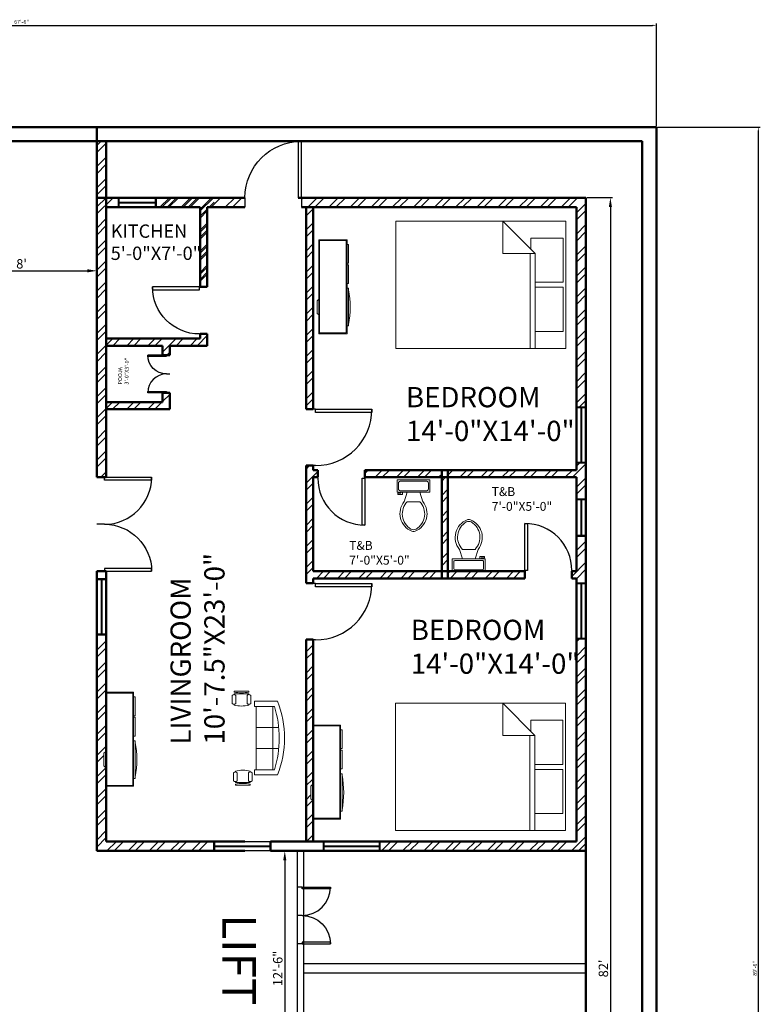
# Model space of a CAD drawing. Units: inches. Extents: x -12550 to 6516, y 1273 to 18700.
# Tile 11 of 19: x 3538 to 4010, y 1958 to 2587. Entities that reach past the tile are written whole.
import ezdxf

# ---------------------------------------------------------------- set-up
doc = ezdxf.new("R2010")
doc.units = ezdxf.units.IN
for name, color, linetype, lineweight in [('A-ANNO-DIMS', 2, 'Continuous', 18), ('A-AREA-IDEN', 1, 'Continuous', 18), ('A-DOOR', 5, 'Continuous', 25), ('A-EQPM', 4, 'Continuous', 25), ('A-FURN', 8, 'Continuous', 18), ('A-GLAZ', 3, 'Continuous', 25), ('A-WALL', 7, 'Continuous', 50), ('A-WALL-PATT', 8, 'Continuous', 13)]:
    doc.layers.add(name, color=color, linetype=linetype, lineweight=lineweight)
doc.styles.get("Standard").update_dxf_attribs({"font": 'arial.ttf'})
doc.dimstyles.new('ISO-25', dxfattribs={"dimtxt": 2.5, "dimasz": 2.5, "dimexe": 1.25, "dimexo": 0.625, "dimtad": 1, "dimlunit": 4, "dimtxsty": 'Standard', "dimcen": 2.5, "dimadec": 0, "dimazin": 0, "dimtfac": 1, "dimtmove": 0, "dimatfit": 3, "dimfxl": 1, "dimarcsym": 0})
pattern_1 = [(45, (1161.5385, 0), (-6.735192, 6.735192), []), (45, (1166.029, 0), (-6.735192, 6.735192), [])]
pattern_2 = [(45, (1161.5385, 567), (-6.735192, 6.735192), []), (45, (1166.029, 567), (-6.735192, 6.735192), [])]

# ---------------------------------------------------------------- blocks, each defined once
blk = doc.blocks.new('*U2')
for p, q in [((0, 0), (0, -5)), ((30, 0), (30, -5))]:
    blk.add_line(p, q)
blk.add_lwpolyline([(0, 0), (0, 30), (1.75, 30), (1.75, 0)], close=True)
blk.add_arc((0, 0), 30, 0, 90)
blk = doc.blocks.new('Bed - Queen')
for p, q in [((0, -80.00003), (0, 0)), ((0, 0), (59.99999, 0)), ((59.99999, 0), (59.99999, -80.00003)), ((7.99999, -1.2), (28.79998, -1.2)), ((7.99999, -14.4), (7.99999, -1.2)), ((28.79998, -1.2), (28.79998, -14.4)), ((31.19999, -1.2), (51.99999, -1.2)), ((31.19999, -14.4), (31.19999, -1.2)), ((51.99999, -1.2), (51.99999, -16.4)), ((0, -14.4), (44.8, -14.4)), ((44.8, -16.8), (0, -16.8)), ((59.99999, -29.6), (44.8, -14.4)), ((44.8, -14.4), (44.8, -29.6)), ((51.99999, -16.4), (46.79936, -16.4)), ((44.8, -29.6), (59.99999, -29.6)), ((59.99999, -80.00003), (0, -80.00003))]:
    blk.add_line(p, q)
blk = doc.blocks.new('Toilet - top')
for p, q in [((9.5, -6), (9.5, -2)), ((-10, -8.5), (-8, -8.5)), ((-10, -9.5), (-10, -8.5)), ((-7, -9.5), (-10, -9.5)), ((-8, -8.5), (-8, -8)), ((-7, -8), (-7, -9.5)), ((-4, -8), (-6, -14)), ((4, -8), (6, -14)), ((4, -14), (-4, -14))]:
    blk.add_line(p, q)
blk.add_lwpolyline([(10.5, -8), (10.5, 0), (-10.5, 0), (-10.5, -8)], close=True)
for points in [[(-9.5, -2), (-9.5, -6)], [(8.5, -1), (-8.5, -1)], [(-8.5, -7), (8.5, -7)]]:
    blk.add_lwpolyline(points)
for centre, radius, start, end in [((-8.62, -1.88), 0.884, 81.8699, 188.1301), ((-8.62, -6.12), 0.884, 171.8699, 278.1301), ((8.62, -1.88), 0.884, 351.8699, 98.1301), ((8.62, -6.12), 0.884, 261.8699, 8.1301), ((3.52, -21.58), 12.17, 141.46911, 247.97143), ((4.2, -21.82), 11.33, 136.36773, 238.94682), ((-3.52, -21.58), 12.17, 292.02843, 38.53071), ((-4.2, -21.82), 11.33, 301.05301, 43.63209), ((0, -27.88), 4, 245.73182, 294.26817), ((0, -29), 4, 254.86053, 285.13947)]:
    blk.add_arc(centre, radius, start, end)
blk = doc.blocks.new('Entertainment Center')
for p, q in [((-4, 0), (-5, -1)), ((4, 0), (-4, 0)), ((5, -1), (4, 0)), ((-17, -19), (-17, -1)), ((-17, -1), (43, -1)), ((-16.5, -18.5), (-16.5, -1.5)), ((-16.5, -1.5), (42.5, -1.5)), ((42.5, -1.5), (42.5, -18.5)), ((43, -1), (43, -19)), ((42.5, -18.5), (-16.5, -18.5)), ((43, -19), (-17, -19)), ((-12, -20), (-12, -19)), ((12, -20), (-12, -20)), ((12, -19), (12, -20)), ((15, -20), (15, -19)), ((27, -20), (15, -20)), ((27, -19), (27, -20)), ((28, -20), (28, -19)), ((40, -20), (28, -20)), ((40, -19), (40, -20))]:
    blk.add_line(p, q)
blk.add_arc((0, 40), 61, 259.6111, 280.3889)
blk = doc.blocks.new('Sofa - Roundback 7 ft.')
for p, q in [((-12.00002, -32.4421), (-12.00003, -6.5971)), ((11.99997, -32.4421), (11.99998, -6.5971)), ((-36.000027, -34), (-36.000027, -11.4696)), ((-35.999844, -13.3819), (35.9998, -13.3819)), ((35.99998, -34), (35.99998, -11.4696)), ((-36.000027, -32.4421), (35.99998, -32.4421))]:
    blk.add_line(p, q)
for points in [[(-36.000027, -34), (-42.000027, -34), (-42.000027, -8)], [(41.99998, -8), (41.99998, -34), (35.99998, -34)]]:
    blk.add_lwpolyline(points)
for centre, radius, start, end in [((0, -114.25), 114.25, 68.43141, 111.5686), ((-0.00001, -127.1968), 121.1968, 72.72033, 107.2797)]:
    blk.add_arc(centre, radius, start, end)
blk = doc.blocks.new('Chair - Desk')
for p, q in [((-8.5, 0), (-8.5, -1)), ((-8.5, 0), (8.5, 0)), ((8.5, 0), (8.5, -1)), ((-10.5, -5), (-10.5, -14)), ((-8.5, -3), (-8.5, -4)), ((-8.5, -3), (8.5, -3)), ((-6.5, -14), (-6.5, -5)), ((-2, -3), (-2, -1.9355)), ((2, -1.9576), (2, -3)), ((6.5, -5), (6.5, -14)), ((8.5, -3), (8.5, -4)), ((10.5, -14), (10.5, -5)), ((-8.5, -15), (-8.5, -16)), ((8.5, -15), (8.5, -16))]:
    blk.add_line(p, q)
for centre, radius, start, end in [((-8.5, -6.5), 2.5, 36.8699, 143.1301), ((0, 34.625), 36.625, 256.5803, 283.4197), ((8.5, -6.5), 2.5, 36.8699, 143.1301), ((-8.5, -12.5), 2.5, 216.8699, 323.1301), ((0, 19.625), 36.625, 256.5803, 283.4197), ((8.5, -12.5), 2.5, 216.8699, 323.1301)]:
    blk.add_arc(centre, radius, start, end)
blk = doc.blocks.new('*D28')
at = {"layer": 'A-ANNO-DIMS', "color": 0, "lineweight": -2, "transparency": 16777216}
for p, q in [((3714.6, 2056.25), (3705.89, 2056.25)), ((3707.14, 2050.25), (3707.14, 1912.25)), ((3714.6, 1906.25), (3705.89, 1906.25))]:
    blk.add_line(p, q, dxfattribs=at)
at = {"layer": 'A-ANNO-DIMS', "color": 0, "transparency": 16777216}
for points in [[(3706.14, 2050.25), (3708.14, 2050.25), (3707.14, 2056.25)], [(3706.14, 1912.25), (3708.14, 1912.25), (3707.14, 1906.25)]]:
    blk.add_solid(points, dxfattribs=at)
at = {"layer": 'Defpoints', "color": 0, "transparency": 16777216}
for p in [(3715.23, 2056.25), (3707.14, 1906.25), (3715.23, 1906.25)]:
    blk.add_point(p, dxfattribs=at)
at = {"layer": 'A-ANNO-DIMS', "color": 0, "transparency": 16777216, "insert": (3703.45, 1981.25), "char_height": 6, "attachment_point": 5, "rotation": 90}
blk.add_mtext('12\'-6"', dxfattribs=at)
blk = doc.blocks.new('*D30')
at = {"layer": 'A-ANNO-DIMS', "color": 0, "lineweight": -2, "transparency": 16777216}
for p, q in [((3899.85, 2473.25), (3916.1, 2473.25)), ((3914.85, 2467.25), (3914.85, 1495.25)), ((3899.85, 1489.25), (3916.1, 1489.25))]:
    blk.add_line(p, q, dxfattribs=at)
at = {"layer": 'A-ANNO-DIMS', "color": 0, "transparency": 16777216}
for points in [[(3913.85, 2467.25), (3915.85, 2467.25), (3914.85, 2473.25)], [(3913.85, 1495.25), (3915.85, 1495.25), (3914.85, 1489.25)]]:
    blk.add_solid(points, dxfattribs=at)
at = {"layer": 'Defpoints', "color": 0, "transparency": 16777216}
for p in [(3899.23, 2473.25), (3899.23, 1489.25), (3914.85, 1489.25)]:
    blk.add_point(p, dxfattribs=at)
at = {"layer": 'A-ANNO-DIMS', "color": 0, "transparency": 16777216, "insert": (3911.16, 1981.25), "char_height": 6, "attachment_point": 5, "rotation": 90}
blk.add_mtext("82'", dxfattribs=at)
blk = doc.blocks.new('*D27')
at = {"layer": 'A-ANNO-DIMS', "color": 0, "lineweight": -2, "transparency": 16777216}
for p, q in [((3491.23, 2407.12), (3491.23, 2427.81)), ((3497.23, 2426.56), (3581.23, 2426.56)), ((3587.23, 2407.12), (3587.23, 2427.81))]:
    blk.add_line(p, q, dxfattribs=at)
at = {"layer": 'A-ANNO-DIMS', "color": 0, "transparency": 16777216}
for points in [[(3497.23, 2427.56), (3497.23, 2425.56), (3491.23, 2426.56)], [(3581.23, 2427.56), (3581.23, 2425.56), (3587.23, 2426.56)]]:
    blk.add_solid(points, dxfattribs=at)
at = {"layer": 'Defpoints', "color": 0, "transparency": 16777216}
for p in [(3587.23, 2426.56), (3491.23, 2406.5), (3587.23, 2406.5)]:
    blk.add_point(p, dxfattribs=at)
at = {"layer": 'A-ANNO-DIMS', "color": 0, "transparency": 16777216, "insert": (3539.23, 2430.25), "char_height": 6, "attachment_point": 5}
blk.add_mtext("8'", dxfattribs=at)
blk = doc.blocks.new('WIN-3FT')
for p, q in [((0, 0), (0, 6)), ((0, 6), (36.02, 6)), ((36.02, 0), (0, 0)), ((0.5, 0), (0.5, 6)), ((35.52, 3.2), (0.5, 3.2)), ((35.52, 2.8), (0.5, 2.8)), ((35.52, 6), (35.52, 0)), ((36.02, 6), (36.02, 0))]:
    blk.add_line(p, q)
blk = doc.blocks.new('WIN-2FT')
for p, q in [((0, 0), (0, 24.02)), ((0, 24.02), (6, 24.02)), ((0, 23.52), (6, 23.52)), ((2.8, 0.5), (2.8, 23.52)), ((3.2, 0.5), (3.2, 23.52)), ((6, 24.02), (6, 0)), ((6, 0.5), (0, 0.5)), ((6, 0), (0, 0))]:
    blk.add_line(p, q)
blk = doc.blocks.new('*D103')
at = {"layer": 'A-ANNO-DIMS', "color": 0, "lineweight": -2, "transparency": 16777216}
for p, q in [((3134.23, 2518.87), (3134.23, 2584.5)), ((3136.73, 2583.25), (3941.73, 2583.25)), ((3944.23, 2518.87), (3944.23, 2584.5))]:
    blk.add_line(p, q, dxfattribs=at)
at = {"layer": 'A-ANNO-DIMS', "color": 0, "transparency": 16777216}
for points in [[(3136.73, 2583.66), (3136.73, 2582.83), (3134.23, 2583.25)], [(3941.73, 2583.66), (3941.73, 2582.83), (3944.23, 2583.25)]]:
    blk.add_solid(points, dxfattribs=at)
at = {"layer": 'Defpoints', "color": 0, "transparency": 16777216}
for p in [(3944.23, 2583.25), (3134.23, 2518.25), (3944.23, 2518.25)]:
    blk.add_point(p, dxfattribs=at)
at = {"layer": 'A-ANNO-DIMS', "color": 0, "transparency": 16777216, "insert": (3539.23, 2585.15), "char_height": 2.5, "attachment_point": 5}
blk.add_mtext('67\'-6"', dxfattribs=at)
blk = doc.blocks.new('*D104')
at = {"layer": 'A-ANNO-DIMS', "color": 0, "lineweight": -2, "transparency": 16777216}
for p, q in [((3944.85, 2518.25), (4010.48, 2518.25)), ((4009.23, 1446.75), (4009.23, 2515.75)), ((3944.85, 1444.25), (4010.48, 1444.25))]:
    blk.add_line(p, q, dxfattribs=at)
at = {"layer": 'A-ANNO-DIMS', "color": 0, "transparency": 16777216}
for points in [[(4008.81, 2515.75), (4009.64, 2515.75), (4009.23, 2518.25)], [(4008.81, 1446.75), (4009.64, 1446.75), (4009.23, 1444.25)]]:
    blk.add_solid(points, dxfattribs=at)
at = {"layer": 'Defpoints', "color": 0, "transparency": 16777216}
for p in [(3944.23, 2518.25), (4009.23, 2518.25), (3944.23, 1444.25)]:
    blk.add_point(p, dxfattribs=at)
at = {"layer": 'A-ANNO-DIMS', "color": 0, "transparency": 16777216, "insert": (4007.33, 1981.25), "char_height": 2.5, "attachment_point": 5, "rotation": 90}
blk.add_mtext('89\'-6"', dxfattribs=at)

msp = doc.modelspace()

# ---------------------------------------------------------------- hatches: boundary and pattern name
at = {"layer": 'A-WALL-PATT'}
h = msp.add_hatch(dxfattribs=at)
h.set_pattern_fill('ANSI32', color=256)
h.set_pattern_definition(pattern_1)
h.paths.add_polyline_path([(3593.227, 2509.247), (3587.227, 2509.247), (3587.227, 2473.247), (3593.227, 2473.247)])
h = msp.add_hatch(dxfattribs=at)
h.set_pattern_fill('ANSI32', color=256)
h.set_pattern_definition(pattern_2)
h.paths.add_polyline_path([(3600.985, 2473.247), (3587.227, 2473.247), (3587.227, 2294.747), (3592.227, 2294.747), (3593.227, 2294.747), (3593.227, 2467.247), (3600.985, 2467.247)])
h = msp.add_hatch(dxfattribs=at)
h.set_pattern_fill('ANSI32', color=256)
h.set_pattern_definition(pattern_1)
h.paths.add_polyline_path([(3625.002, 2473.247), (3625.002, 2467.247), (3653.227, 2467.247), (3653.227, 2416.247), (3657.727, 2416.247), (3657.727, 2467.247), (3681.727, 2467.247), (3681.727, 2473.247)])
h = msp.add_hatch(dxfattribs=at)
h.set_pattern_fill('ANSI32', color=256)
h.set_pattern_definition(pattern_2)
h.paths.add_polyline_path([(3662.066, 2473.247), (3625.002, 2473.247), (3625.002, 2467.247), (3653.227, 2467.247), (3653.227, 2416.247), (3657.727, 2416.247), (3657.727, 2467.247), (3662.066, 2467.247)])
h = msp.add_hatch(dxfattribs=at)
h.set_pattern_fill('ANSI32', color=256)
h.set_pattern_definition(pattern_2)
h.paths.add_polyline_path([(3717.727, 2473.247), (3717.727, 2467.247), (3893.227, 2467.247), (3893.227, 2339.747), (3899.227, 2339.747), (3899.227, 2473.247)])
h = msp.add_hatch(dxfattribs=at)
h.set_pattern_fill('ANSI32', color=256)
h.set_pattern_definition(pattern_2)
h.paths.add_polyline_path([(3725.227, 2467.247), (3720.727, 2467.247), (3720.727, 2338.247), (3725.227, 2338.247)])
h = msp.add_hatch(dxfattribs=at)
h.set_pattern_fill('ANSI32', color=256)
h.set_pattern_definition(pattern_2)
h.paths.add_polyline_path([(3657.727, 2386.247), (3653.227, 2386.247), (3653.227, 2383.247), (3593.227, 2383.247), (3593.227, 2378.747), (3629.227, 2378.747), (3629.227, 2372.747), (3631.727, 2372.747), (3633.727, 2372.747), (3633.727, 2378.747), (3657.727, 2378.747)])
h = msp.add_hatch(dxfattribs=at)
h.set_pattern_fill('ANSI32', color=256)
h.set_pattern_definition(pattern_2)
h.paths.add_polyline_path([(3633.727, 2348.747), (3631.727, 2348.747), (3629.227, 2348.747), (3629.227, 2342.747), (3593.227, 2342.747), (3593.227, 2338.247), (3633.727, 2338.247)])
h = msp.add_hatch(dxfattribs=at)
h.set_pattern_fill('ANSI32', color=256)
h.set_pattern_definition(pattern_2)
h.paths.add_polyline_path([(3725.227, 2294.747), (3728.227, 2294.747), (3728.227, 2299.247), (3725.227, 2299.247), (3725.227, 2302.247), (3720.727, 2302.247), (3720.727, 2227.247), (3725.227, 2227.247), (3725.227, 2230.247), (3728.18, 2230.247), (3807.227, 2230.247), (3807.227, 2234.747), (3728.18, 2234.747), (3725.227, 2234.747)])
h = msp.add_hatch(dxfattribs=at)
h.set_pattern_fill('ANSI32', color=256)
h.set_pattern_definition(pattern_2)
h.paths.add_polyline_path([(3899.227, 2303.73), (3893.227, 2303.73), (3893.227, 2299.247), (3890.227, 2299.247), (3811.227, 2299.247), (3811.227, 2294.747), (3890.227, 2294.747), (3893.227, 2294.747), (3893.227, 2281.042), (3899.227, 2281.042)])
h = msp.add_hatch(dxfattribs=at)
h.set_pattern_fill('ANSI32', color=256)
h.set_pattern_definition(pattern_2)
h.paths.add_polyline_path([(3807.227, 2299.247), (3758.227, 2299.247), (3758.227, 2294.747), (3807.227, 2294.747)], flags=17)
h = msp.add_hatch(dxfattribs=at)
h.set_pattern_fill('ANSI32', color=256)
h.set_pattern_definition(pattern_2)
h.paths.add_polyline_path([(3811.227, 2294.747), (3807.227, 2294.747), (3807.227, 2234.747), (3811.227, 2234.747)])
h = msp.add_hatch(dxfattribs=at)
h.set_pattern_fill('ANSI32', color=256)
h.set_pattern_definition(pattern_2)
h.paths.add_polyline_path([(3899.227, 2257.024), (3893.227, 2257.024), (3893.227, 2234.747), (3890.227, 2234.747), (3890.227, 2230.247), (3893.227, 2230.247), (3893.227, 2227.369), (3899.227, 2227.369)])
h = msp.add_hatch(dxfattribs=at)
h.set_pattern_fill('ANSI32', color=256)
h.set_pattern_definition(pattern_2)
h.paths.add_polyline_path([(3860.227, 2234.747), (3811.227, 2234.747), (3811.227, 2230.247), (3860.227, 2230.247)])
h = msp.add_hatch(dxfattribs=at)
h.set_pattern_fill('ANSI32', color=256)
h.set_pattern_definition(pattern_2)
h.paths.add_polyline_path([(3662.066, 2056.247), (3662.066, 2062.247), (3593.227, 2062.247), (3593.227, 2097.559), (3592.727, 2097.559), (3592.727, 2109.559), (3591.727, 2110.559), (3591.727, 2118.559), (3592.727, 2119.559), (3592.727, 2157.559), (3593.227, 2157.559), (3593.227, 2194.032), (3587.227, 2194.032), (3587.227, 2056.247)])
h = msp.add_hatch(dxfattribs=at)
h.set_pattern_fill('ANSI32', color=256)
h.set_pattern_definition(pattern_2)
h.paths.add_polyline_path([(3720.727, 2190.947), (3720.727, 2062.247), (3725.227, 2062.247), (3725.227, 2076.575), (3724.727, 2076.575), (3724.727, 2088.575), (3723.727, 2089.575), (3723.727, 2097.575), (3724.727, 2098.575), (3724.727, 2136.575), (3725.225, 2190.947)])
h = msp.add_hatch(dxfattribs=at)
h.set_pattern_fill('ANSI32', color=256)
h.set_pattern_definition(pattern_2)
h.paths.add_polyline_path([(3899.227, 2191.352), (3893.227, 2191.352), (3893.227, 2062.247), (3767.813, 2062.247), (3767.813, 2056.247), (3899.227, 2056.247)])

# ---------------------------------------------------------------- linework, layer by layer
at = {"layer": 'A-EQPM'}
for p, q in [((3715.227, 1906.247), (3715.227, 2056.247)), ((3899.227, 2056.247), (3715.227, 2056.247)), ((3719.227, 1906.247), (3719.227, 2056.247)), ((3899.227, 2056.247), (3899.227, 1906.247)), ((3899.227, 1984.247), (3719.227, 1984.247)), ((3899.227, 1978.247), (3719.227, 1978.247))]:
    msp.add_line(p, q, dxfattribs=at)
at = {"layer": 'A-WALL'}
for p, q in [((3134.227, 2518.247), (3944.227, 2518.247)), ((3587.227, 2294.747), (3587.227, 2518.247)), ((3944.227, 2518.247), (3944.227, 1444.247)), ((3143.227, 2509.247), (3935.227, 2509.247)), ((3715.627, 2509.247), (3415.627, 2509.247)), ((3593.227, 2294.747), (3593.227, 2509.247)), ((3935.227, 2509.247), (3935.227, 1453.247)), ((3681.727, 2473.247), (3587.227, 2473.247)), ((3720.727, 2473.247), (3715.627, 2473.247)), ((3899.227, 2473.247), (3720.727, 2473.247)), ((3899.227, 2060.923), (3899.227, 2473.247)), ((3653.227, 2467.247), (3593.227, 2467.247)), ((3653.227, 2416.247), (3653.227, 2467.247)), ((3681.727, 2467.247), (3657.727, 2467.247)), ((3657.727, 2416.247), (3657.727, 2467.247)), ((3720.727, 2467.247), (3717.727, 2467.247)), ((3893.227, 2467.247), (3720.727, 2467.247)), ((3720.727, 2338.247), (3720.727, 2467.247)), ((3725.227, 2338.247), (3725.227, 2467.247)), ((3893.227, 2299.247), (3893.227, 2467.247)), ((3653.227, 2416.247), (3657.727, 2416.247)), ((3653.227, 2383.247), (3593.227, 2383.247)), ((3653.227, 2383.247), (3653.227, 2386.247)), ((3657.727, 2386.247), (3653.227, 2386.247)), ((3657.727, 2378.747), (3657.727, 2386.247)), ((3657.727, 2383.247), (3657.727, 2386.247)), ((3629.227, 2378.747), (3593.227, 2378.747)), ((3629.227, 2372.747), (3629.227, 2378.747)), ((3657.727, 2378.747), (3633.727, 2378.747)), ((3633.727, 2372.747), (3633.727, 2378.747)), ((3629.227, 2372.747), (3633.727, 2372.747)), ((3629.227, 2342.747), (3629.227, 2348.747)), ((3633.727, 2348.747), (3629.227, 2348.747)), ((3633.727, 2338.247), (3633.727, 2348.747)), ((3633.727, 2342.747), (3633.727, 2348.747)), ((3629.227, 2342.747), (3593.227, 2342.747)), ((3633.727, 2338.247), (3593.227, 2338.247)), ((3720.727, 2338.247), (3725.227, 2338.247)), ((3720.727, 2227.247), (3720.727, 2302.247)), ((3725.227, 2302.247), (3720.727, 2302.247)), ((3725.227, 2299.247), (3725.227, 2302.247)), ((3725.227, 2299.247), (3725.227, 2302.247)), ((3725.227, 2299.247), (3725.227, 2302.247)), ((3725.227, 2299.247), (3725.227, 2302.247)), ((3593.227, 2294.747), (3587.227, 2294.747)), ((3728.227, 2299.247), (3725.227, 2299.247)), ((3728.227, 2294.747), (3725.227, 2294.747)), ((3725.227, 2234.747), (3725.227, 2294.747)), ((3725.227, 2234.747), (3725.227, 2294.747)), ((3725.227, 2234.747), (3725.227, 2294.747)), ((3725.227, 2294.747), (3728.227, 2294.747)), ((3728.227, 2294.747), (3728.227, 2299.247)), ((3890.227, 2299.247), (3758.227, 2299.247)), ((3758.227, 2299.247), (3758.227, 2294.747)), ((3890.227, 2294.747), (3758.227, 2294.747)), ((3807.227, 2230.247), (3807.227, 2299.247)), ((3811.227, 2230.247), (3811.227, 2299.247)), ((3893.227, 2299.247), (3890.227, 2299.247)), ((3893.227, 2299.247), (3890.227, 2299.247)), ((3893.227, 2294.747), (3890.227, 2294.747)), ((3893.227, 2234.747), (3893.227, 2294.747)), ((3593.227, 2234.747), (3587.227, 2234.747)), ((3587.227, 2056.247), (3587.227, 2234.747)), ((3593.227, 2062.247), (3593.227, 2234.747)), ((3728.18, 2234.747), (3725.227, 2234.747)), ((3860.227, 2234.747), (3728.18, 2234.747)), ((3860.227, 2234.747), (3860.227, 2230.247)), ((3893.227, 2234.747), (3890.227, 2234.747)), ((3890.227, 2230.247), (3890.227, 2234.747)), ((3720.727, 2230.247), (3720.727, 2227.247)), ((3720.727, 2227.247), (3725.227, 2227.247)), ((3728.18, 2230.247), (3725.227, 2230.247)), ((3725.227, 2227.247), (3725.227, 2230.247)), ((3725.227, 2227.247), (3725.227, 2230.247)), ((3725.227, 2227.247), (3725.227, 2230.247)), ((3860.227, 2230.247), (3728.18, 2230.247)), ((3893.227, 2230.247), (3890.227, 2230.247)), ((3893.227, 2230.247), (3890.227, 2230.247)), ((3893.227, 2062.247), (3893.227, 2230.247)), ((3720.727, 2062.247), (3720.727, 2191.247)), ((3725.227, 2191.247), (3720.727, 2191.247)), ((3725.227, 2062.247), (3725.227, 2191.247)), ((3681.727, 2062.247), (3593.227, 2062.247)), ((3662.066, 2062.247), (3662.066, 2056.247)), ((3698.084, 2062.247), (3698.084, 2056.247)), ((3717.727, 2062.247), (3698.084, 2062.247)), ((3893.227, 2062.247), (3717.727, 2062.247)), ((3720.727, 2062.247), (3717.727, 2062.247)), ((3681.727, 2056.247), (3587.227, 2056.247)), ((3698.084, 2056.247), (3717.727, 2056.247)), ((3899.227, 2056.247), (3717.727, 2056.247)), ((3899.227, 1489.247), (3899.227, 2060.923)), ((3935.227, 1489.247), (3935.227, 2060.923))]:
    msp.add_line(p, q, dxfattribs=at)

# ---------------------------------------------------------------- block references
at = {"layer": 'A-DOOR', "xscale": -1.199999999999999, "yscale": 1.199999999999999, "zscale": 1.199999999999999}
msp.add_blockref('*U2', (3717.727, 2473.247), dxfattribs=at)
at = {"layer": 'A-DOOR', "xscale": -1}
for p, rotation in [((3652.727, 2416.247), 90), ((3592.227, 2234.747), 270)]:
    msp.add_blockref('*U2', p, dxfattribs=dict(at, rotation=rotation))
at = {"layer": 'A-DOOR'}
for p, xscale, yscale, zscale, rotation in [((3631.727, 2372.747), -0.399999999999997, 0.399999999999997, 0.399999999999997, 90), ((3631.727, 2348.747), 0.399999999999997, 0.399999999999997, 0.399999999999997, 90.00000000000003), ((3726.727, 2338.247), 1.199999999999999, 1.199999999999999, 1.199999999999999, 270), ((3726.727, 2226.947), 1.199999999999999, 1.199999999999999, 1.199999999999999, 270)]:
    msp.add_blockref('*U2', p, dxfattribs=dict(at, xscale=xscale, yscale=yscale, zscale=zscale, rotation=rotation))
for p, rotation in [((3592.227, 2294.747), 270), ((3758.227, 2294.247), 180)]:
    msp.add_blockref('*U2', p, dxfattribs=dict(at, rotation=rotation))
msp.add_blockref('*U2', (3860.227, 2235.247), dxfattribs=at)
at = {"layer": 'A-EQPM', "yscale": 0.5999999999999954, "zscale": 0.5999999999999954, "rotation": 270}
for p, xscale in [((3718.227, 2033.042), 0.5999999999999954), ((3718.227, 1997.042), -0.5999999999999954)]:
    msp.add_blockref('*U2', p, dxfattribs=dict(at, xscale=xscale))
at = {"layer": 'A-FURN'}
for name, p, xscale, yscale, zscale, rotation in [('Bed - Queen', (3886.407, 2376.994), -1.354827908062564, 1.354827908062564, 1.354827908062564, 270), ('Sofa - Roundback 7 ft.', (3706.946, 2128.265), 0.5595223685495907, 0.5595223685495907, 0.5595223685495907, 270), ('Bed - Queen', (3886.246, 2069.217), -1.354827908062564, 1.354827908062564, 1.354827908062564, 270), ('Chair - Desk', (3680.361, 2098.281), 0.5595223685495907, 0.5595223685495907, 0.5595223685495907, 180)]:
    msp.add_blockref(name, p, dxfattribs=dict(at, xscale=xscale, yscale=yscale, zscale=zscale, rotation=rotation))
for name, p, rotation in [('Entertainment Center', (3727.857, 2403.379), 89.99999999999999), ('Toilet - top', (3824.496, 2234.747), 180), ('Entertainment Center', (3591.727, 2114.559), 89.99999999999999), ('Entertainment Center', (3723.727, 2093.575), 89.99999999999999)]:
    msp.add_blockref(name, p, dxfattribs=dict(at, rotation=rotation))
msp.add_blockref('Toilet - top', (3789.25, 2293.198), dxfattribs=at)
at = {"layer": 'A-FURN', "xscale": 0.5595223685495907, "yscale": 0.5595223685495907, "zscale": 0.5595223685495907}
msp.add_blockref('Chair - Desk', (3679.507, 2158.265), dxfattribs=at)
at = {"layer": 'A-GLAZ'}
for name, p, rotation in [('WIN-2FT', (3600.984, 2473.247), 269.9999999999969), ('WIN-3FT', (3899.228, 2303.73), 90.00000000000351), ('WIN-2FT', (3899.227, 2281.042), 180), ('WIN-3FT', (3593.228, 2194.032), 90.00000000000047), ('WIN-3FT', (3899.228, 2191.352), 90.0000000000033), ('WIN-3FT', (3698.083, 2062.247), 180), ('WIN-3FT', (3767.813, 2062.247), 180)]:
    msp.add_blockref(name, p, dxfattribs=dict(at, rotation=rotation))

# ---------------------------------------------------------------- texts
at = {"layer": 'A-AREA-IDEN', "attachment_point": 1}
for s, width, gutter_width, insert, char_height in [('KITCHEN\\P5\'-0"X7\'-0"', 1.29487, 42.422, (3596.107, 2456.124), 8.48435), ('T&B\\P7\'-0"X5\'-0"', 4.19569, 28.328, (3839.149, 2288.465), 5.66556), ('T&B\\P7\'-0"X5\'-0"', 4.19569, 28.328, (3748.24, 2254.107), 5.66556)]:
    msp.add_mtext_dynamic_manual_height_columns(s, width=width, gutter_width=gutter_width, heights=[0], dxfattribs=dict(at, insert=insert, char_height=char_height))
for s, width, gutter_width, insert, char_height, rotation in [('POOJA\\P3\'-0"X3\'-0"', 0.78585, 12.5, (3600.779, 2354.026), 2.5, 89.183853), ('LIFT', 3.27433, 107.272, (3688.715, 2015.823), 21.4543, 270)]:
    msp.add_mtext_dynamic_manual_height_columns(s, width=width, gutter_width=gutter_width, heights=[0], dxfattribs=dict(at, insert=insert, char_height=char_height, rotation=rotation))
at = {"layer": 'A-AREA-IDEN', "char_height": 12.93169, "attachment_point": 1}
for insert in [(3784.442, 2352.378), (3787.508, 2203.812)]:
    msp.add_mtext('BEDROOM\\P14\'-0"X14\'-0"', dxfattribs=dict(at, insert=insert))
at = {"layer": 'A-AREA-IDEN', "insert": (3634.251, 2124.153), "char_height": 12.93169, "attachment_point": 1, "rotation": 90}
msp.add_mtext('LIVINGROOM\\P10\'-7.5"X23\'-0"', dxfattribs=at)

# ---------------------------------------------------------------- dimensions: what is measured, and where the dimension line sits
at = {"layer": 'A-ANNO-DIMS'}
for base, p1, p2, override, picture, middle in [((3944.227, 2583.247), (3134.227, 2518.247), (3944.227, 2518.247), {"dimdec": 1, "dimlfac": 1, "dimrnd": 0, "dimzin": 1, "dimdsep": 46, "dimlunit": 4, "dimfrac": 2}, '*D103', (3539.227, 2585.149)), ((3587.227, 2426.562), (3491.227, 2406.497), (3587.227, 2406.497), {"dimtxt": 6, "dimasz": 6, "dimclrd": 0, "dimclre": 0, "dimclrt": 0}, '*D27', (3539.227, 2430.25))]:
    dim = msp.add_linear_dim(base=base, p1=p1, p2=p2, dimstyle='ISO-25', override=override, dxfattribs=at)
    dim.commit()
    dim.dimension.update_dxf_attribs({"geometry": picture, "text_midpoint": middle})
for base, p1, p2, override, picture, middle in [((4009.227, 2518.247), (3944.227, 1444.247), (3944.227, 2518.247), {"dimdec": 1, "dimlfac": 1, "dimrnd": 0, "dimzin": 1, "dimdsep": 46, "dimlunit": 4, "dimfrac": 2}, '*D104', (4007.326, 1981.247)), ((3914.847, 1489.247), (3899.227, 2473.247), (3899.227, 1489.247), {"dimtxt": 6, "dimasz": 6, "dimclrd": 0, "dimclre": 0, "dimclrt": 0}, '*D30', (3911.159, 1981.247)), ((3707.141, 1906.247), (3715.227, 2056.247), (3715.227, 1906.247), {"dimtxt": 6, "dimasz": 6, "dimclrd": 0, "dimclre": 0, "dimclrt": 0}, '*D28', (3703.452, 1981.247))]:
    dim = msp.add_linear_dim(base=base, p1=p1, p2=p2, angle=90, dimstyle='ISO-25', override=override, dxfattribs=at)
    dim.commit()
    dim.dimension.update_dxf_attribs({"geometry": picture, "text_midpoint": middle})

doc.saveas('drawing.dxf')
